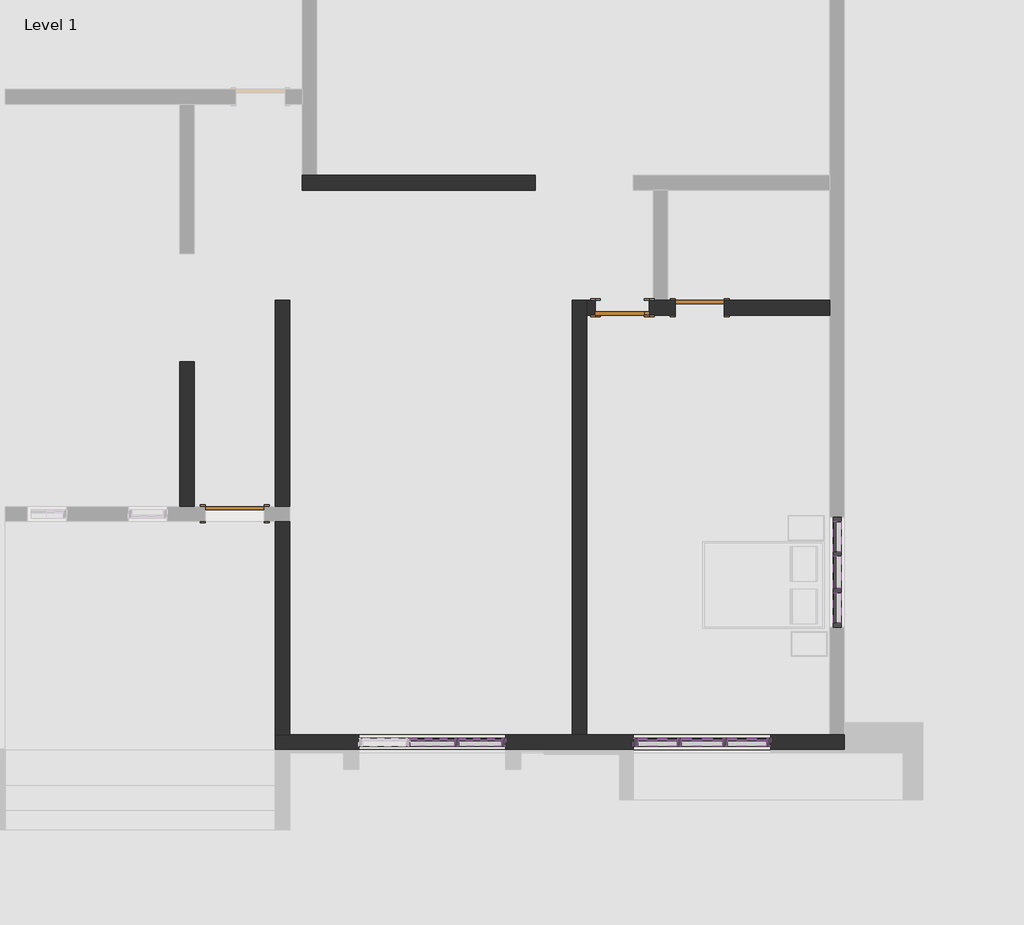
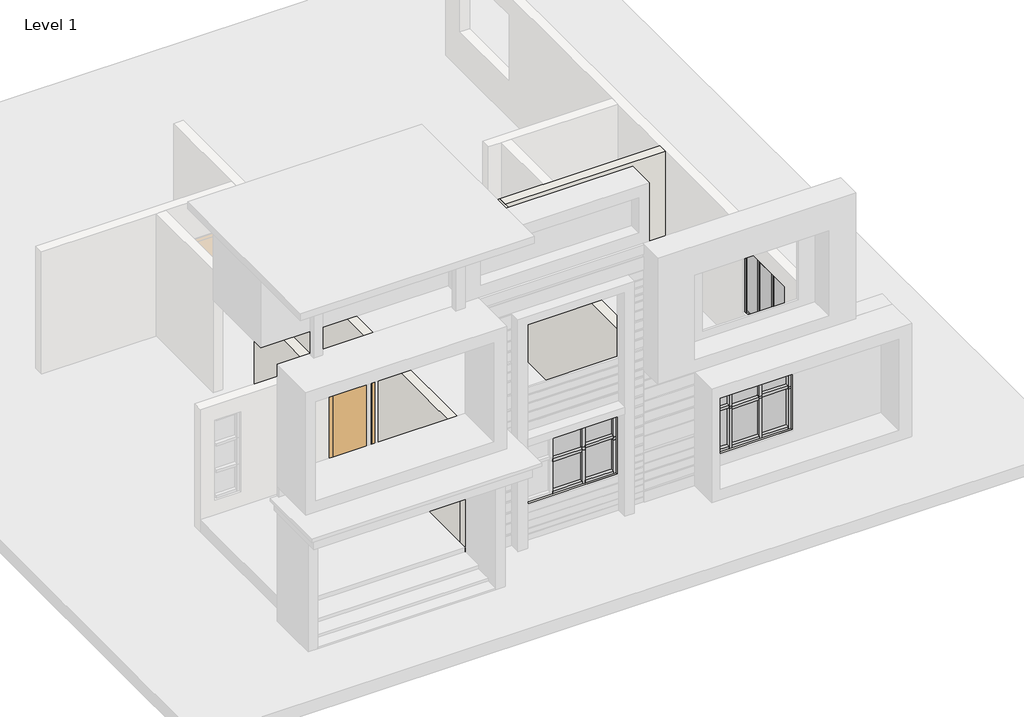
# One storey, part 2 of 3: 43 members, 13 plates, 7 walls, 4 doors.
"""IFC4 building model written with IfcOpenShell, lengths in millimetres."""

from ifc_helpers import new_model, si_unit, origin, origin_with_axes, place, context, project, spatial, polyline, outline, extrude, faceted_brep, transform, mapped, element, save
from components import door_a1484949, door_85036156, door_0ca8825f, member_67dd967c, member_0af91ce1, member_6b0a351e, member_c1cae106, member_3f0e0172, member_5215b92c, member_00d00b53, member_c7c5a8a0, member_eb7364f1, member_b955a9e9, member_5ab2641c, member_2ee2964b, member_c33c434a, member_a6ee1c2c, member_3d7cb871, member_24f36acb, member_06be906d, member_e53b78c9, member_f8dc38bf, member_67d1cd44, member_8f31a534, member_a1cc4565, member_fc709e3d, member_6f38b482, system_panel_glazed_52f1247e, system_panel_glazed_66bb8edf, system_panel_glazed_3a643d3b, system_panel_glazed_b47efb59, system_panel_glazed_21711ca4, system_panel_glazed_687c427d, system_panel_glazed_bb181a04, system_panel_glazed_a28047ed, system_panel_glazed_c0474106, system_panel_glazed_f63241ef

model = new_model("IFC4")

# Units and contexts
model_context = context("Model", 3, world=origin())
ifc_project = project(units=[si_unit("LENGTHUNIT", "METRE", prefix="MILLI")], contexts=[model_context])

# Site, building, storey
site = spatial("IfcSite", under=ifc_project)
building = spatial("IfcBuilding", under=site)
storey = spatial("IfcBuildingStorey", under=building, Name="Level 1", Elevation=0.0)

# Doors
placement = place(None, origin())
door_shape = door_a1484949(model_context)
element("IfcDoor", 1, ObjectType="Single-Flush : 30\" x 80\"", at=placement, inside=storey, context=model_context, shape_type="MappedRepresentation", body=[
    mapped(door_shape, transform((-9027.8261094, -8002.146149, 0.0), x_axis=(-1.0, 0.0, 0.0), y_axis=(0.0, -1.0, 0.0), z_axis=(0.0, 0.0, 1.0))),
])
element("IfcDoor", 2, ObjectType="Single-Flush : 30\" x 80\"", at=placement, inside=storey, context=model_context, shape_type="MappedRepresentation", body=[
    mapped(door_shape, transform((-8951.6261094, -8002.146149, 0.0), x_axis=(-1.0, 0.0, 0.0), y_axis=(0.0, -1.0, 0.0), z_axis=(0.0, 0.0, 1.0))),
])
door_2_shape = door_85036156(model_context)
element("IfcDoor", 3, ObjectType="Single-Flush : 30\" x 80\"", at=placement, inside=storey, context=model_context, shape_type="MappedRepresentation", body=[
    mapped(door_2_shape, transform((-7789.5761094, -8002.146149, 0.0), x_axis=(-1.0, 0.0, 0.0), y_axis=(0.0, -1.0, 0.0), z_axis=(0.0, 0.0, 1.0))),
])
door_3_shape = door_0ca8825f(model_context)
element("IfcDoor", 4, ObjectType="Single-Flush : 36\" x 84\"", at=placement, inside=storey, context=model_context, shape_type="MappedRepresentation", body=[
    mapped(door_3_shape, transform((-15009.5261094, -11202.546149, 355.6), x_axis=(1.0, 0.0, 0.0), y_axis=(0.0, 1.0, 0.0), z_axis=(0.0, 0.0, 1.0))),
])

# Members
member_shape = member_67dd967c(model_context)
element("IfcMember", 5, ObjectType="Rectangular Mullion : 2.5\" x 5\" rectangular", at=placement, inside=storey, context=model_context, shape_type="MappedRepresentation", body=[
    mapped(member_shape, transform((-5655.9761094, -11855.5157064, 2620.512388), x_axis=(0.0, 0.0, 1.0), y_axis=(1.0, 0.0, 0.0), z_axis=(0.0, 1.0, 0.0))),
])
member_2_shape = member_0af91ce1(model_context)
element("IfcMember", 6, ObjectType="Rectangular Mullion : 2.5\" x 5\" rectangular", at=placement, inside=storey, context=model_context, shape_type="MappedRepresentation", body=[
    mapped(member_2_shape, transform((-5655.9761094, -12422.7823731, 2620.512388), x_axis=(0.0, 0.0, 1.0), y_axis=(1.0, 0.0, 0.0), z_axis=(0.0, 1.0, 0.0))),
])
element("IfcMember", 7, ObjectType="Rectangular Mullion : 2.5\" x 5\" rectangular", at=placement, inside=storey, context=model_context, shape_type="MappedRepresentation", body=[
    mapped(member_2_shape, transform((-5655.9761094, -11319.9990397, 2620.512388), x_axis=(0.0, 0.0, 1.0), y_axis=(1.0, 0.0, 0.0), z_axis=(0.0, 1.0, 0.0))),
])
member_3_shape = member_6b0a351e(model_context)
element("IfcMember", 8, ObjectType="Rectangular Mullion : 2.5\" x 5\" rectangular", at=placement, inside=storey, context=model_context, shape_type="MappedRepresentation", body=[
    mapped(member_3_shape, transform((-5655.9761094, -11823.7657064, 945.2248153), x_axis=(0.0, 1.0, 0.0), y_axis=(1.0, 0.0, 0.0), z_axis=(0.0, 0.0, -1.0))),
])
element("IfcMember", 9, ObjectType="Rectangular Mullion : 2.5\" x 5\" rectangular", at=placement, inside=storey, context=model_context, shape_type="MappedRepresentation", body=[
    mapped(member_3_shape, transform((-5655.9761094, -12391.0323731, 945.2248153), x_axis=(0.0, 1.0, 0.0), y_axis=(1.0, 0.0, 0.0), z_axis=(0.0, 0.0, -1.0))),
])
element("IfcMember", 10, ObjectType="Rectangular Mullion : 2.5\" x 5\" rectangular", at=placement, inside=storey, context=model_context, shape_type="MappedRepresentation", body=[
    mapped(member_2_shape, transform((-5655.9761094, -11792.0157064, 945.2248153), x_axis=(0.0, 0.0, -1.0), y_axis=(1.0, 0.0, 0.0), z_axis=(0.0, -1.0, 0.0))),
])
element("IfcMember", 11, ObjectType="Rectangular Mullion : 2.5\" x 5\" rectangular", at=placement, inside=storey, context=model_context, shape_type="MappedRepresentation", body=[
    mapped(member_2_shape, transform((-5655.9761094, -12894.7990397, 945.2248153), x_axis=(0.0, 0.0, -1.0), y_axis=(1.0, 0.0, 0.0), z_axis=(0.0, -1.0, 0.0))),
])
element("IfcMember", 12, ObjectType="Rectangular Mullion : 2.5\" x 5\" rectangular", at=placement, inside=storey, context=model_context, shape_type="MappedRepresentation", body=[
    mapped(member_shape, transform((-5655.9761094, -12359.2823731, 945.2248153), x_axis=(0.0, 0.0, -1.0), y_axis=(1.0, 0.0, 0.0), z_axis=(0.0, -1.0, 0.0))),
])
member_4_shape = member_c1cae106(model_context)
element("IfcMember", 13, ObjectType="Rectangular Mullion : 2.5\" x 5\" rectangular", at=placement, inside=storey, context=model_context, shape_type="MappedRepresentation", body=[
    mapped(member_4_shape, transform((-5655.9761094, -11256.4990397, 945.2248153), x_axis=(0.0, 1.0, 0.0), y_axis=(1.0, 0.0, 0.0), z_axis=(0.0, 0.0, -1.0))),
])
element("IfcMember", 14, ObjectType="Rectangular Mullion : 2.5\" x 5\" rectangular", at=placement, inside=storey, context=model_context, shape_type="MappedRepresentation", body=[
    mapped(member_4_shape, transform((-5655.9761094, -12958.2990397, 2620.512388), x_axis=(0.0, -1.0, 0.0), y_axis=(1.0, 0.0, 0.0), z_axis=(0.0, 0.0, 1.0))),
])
member_5_shape = member_3f0e0172(model_context)
element("IfcMember", 15, ObjectType="Rectangular Mullion : 2.5\" x 5\" rectangular", at=placement, inside=storey, context=model_context, shape_type="MappedRepresentation", body=[
    mapped(member_5_shape, transform((-8139.2627168, -14745.846149, 2528.3677735), x_axis=(0.0, 0.0, 1.0), y_axis=(0.0, -1.0, 0.0), z_axis=(1.0, 0.0, 0.0))),
])
element("IfcMember", 16, ObjectType="Rectangular Mullion : 2.5\" x 5\" rectangular", at=placement, inside=storey, context=model_context, shape_type="MappedRepresentation", body=[
    mapped(member_5_shape, transform((-6748.6127168, -14745.846149, 2528.3677735), x_axis=(0.0, 0.0, 1.0), y_axis=(0.0, -1.0, 0.0), z_axis=(1.0, 0.0, 0.0))),
])
element("IfcMember", 17, ObjectType="Rectangular Mullion : 2.5\" x 5\" rectangular", at=placement, inside=storey, context=model_context, shape_type="MappedRepresentation", body=[
    mapped(member_5_shape, transform((-7364.5627168, -14745.846149, 537.8317429), x_axis=(0.0, 0.0, -1.0), y_axis=(0.0, -1.0, 0.0), z_axis=(-1.0, 0.0, 0.0))),
])
element("IfcMember", 18, ObjectType="Rectangular Mullion : 2.5\" x 5\" rectangular", at=placement, inside=storey, context=model_context, shape_type="MappedRepresentation", body=[
    mapped(member_5_shape, transform((-8755.2127168, -14745.846149, 537.8317429), x_axis=(0.0, 0.0, -1.0), y_axis=(0.0, -1.0, 0.0), z_axis=(-1.0, 0.0, 0.0))),
])
member_6_shape = member_5215b92c(model_context)
element("IfcMember", 19, ObjectType="Rectangular Mullion : 2.5\" x 5\" rectangular", at=placement, inside=storey, context=model_context, shape_type="MappedRepresentation", body=[
    mapped(member_6_shape, transform((-7428.0627168, -14745.846149, 2528.3677735), x_axis=(0.0, 0.0, 1.0), y_axis=(0.0, -1.0, 0.0), z_axis=(1.0, 0.0, 0.0))),
])
element("IfcMember", 20, ObjectType="Rectangular Mullion : 2.5\" x 5\" rectangular", at=placement, inside=storey, context=model_context, shape_type="MappedRepresentation", body=[
    mapped(member_6_shape, transform((-8075.7627168, -14745.846149, 537.8317429), x_axis=(0.0, 0.0, -1.0), y_axis=(0.0, -1.0, 0.0), z_axis=(-1.0, 0.0, 0.0))),
])
member_7_shape = member_00d00b53(model_context)
element("IfcMember", 21, ObjectType="Rectangular Mullion : 2.5\" x 5\" rectangular", at=placement, inside=storey, context=model_context, shape_type="MappedRepresentation", body=[
    mapped(member_7_shape, transform((-11561.9127168, -14745.846149, 1704.2081862), x_axis=(1.0, 0.0, 0.0), y_axis=(0.0, -1.0, 0.0), z_axis=(0.0, 0.0, -1.0))),
])
member_8_shape = member_c7c5a8a0(model_context)
element("IfcMember", 22, ObjectType="Rectangular Mullion : 2.5\" x 5\" rectangular", at=placement, inside=storey, context=model_context, shape_type="MappedRepresentation", body=[
    mapped(member_8_shape, transform((-11593.6627168, -14745.846149, 1704.2081862), x_axis=(0.0, 0.0, 1.0), y_axis=(0.0, -1.0, 0.0), z_axis=(1.0, 0.0, 0.0))),
])
member_9_shape = member_eb7364f1(model_context)
element("IfcMember", 23, ObjectType="Rectangular Mullion : 2.5\" x 5\" rectangular", at=placement, inside=storey, context=model_context, shape_type="MappedRepresentation", body=[
    mapped(member_9_shape, transform((-11561.9127168, -14745.846149, 1780.4081862), x_axis=(1.0, 0.0, 0.0), y_axis=(0.0, -1.0, 0.0), z_axis=(0.0, 0.0, -1.0))),
])
member_10_shape = member_b955a9e9(model_context)
element("IfcMember", 24, ObjectType="Rectangular Mullion : 2.5\" x 5\" rectangular", at=placement, inside=storey, context=model_context, shape_type="MappedRepresentation", body=[
    mapped(member_10_shape, transform((-11593.6627168, -14745.846149, 2536.7442955), x_axis=(0.0, 0.0, 1.0), y_axis=(0.0, -1.0, 0.0), z_axis=(1.0, 0.0, 0.0))),
])
member_11_shape = member_5ab2641c(model_context)
element("IfcMember", 25, ObjectType="Rectangular Mullion : 2.5\" x 5\" rectangular", at=placement, inside=storey, context=model_context, shape_type="MappedRepresentation", body=[
    mapped(member_11_shape, transform((-11561.9127168, -14745.846149, 871.6720769), x_axis=(1.0, 0.0, 0.0), y_axis=(0.0, -1.0, 0.0), z_axis=(0.0, 0.0, -1.0))),
])
element("IfcMember", 26, ObjectType="Rectangular Mullion : 2.5\" x 5\" rectangular", at=placement, inside=storey, context=model_context, shape_type="MappedRepresentation", body=[
    mapped(member_10_shape, transform((-12292.1627168, -14745.846149, 871.6720769), x_axis=(0.0, 0.0, -1.0), y_axis=(0.0, -1.0, 0.0), z_axis=(-1.0, 0.0, 0.0))),
])
member_12_shape = member_2ee2964b(model_context)
element("IfcMember", 27, ObjectType="Rectangular Mullion : 2.5\" x 5\" rectangular", at=placement, inside=storey, context=model_context, shape_type="MappedRepresentation", body=[
    mapped(member_12_shape, transform((-10863.4127168, -14745.846149, 1780.4081862), x_axis=(0.0, 0.0, 1.0), y_axis=(0.0, -1.0, 0.0), z_axis=(1.0, 0.0, 0.0))),
])
member_13_shape = member_c33c434a(model_context)
element("IfcMember", 28, ObjectType="Rectangular Mullion : 2.5\" x 5\" rectangular", at=placement, inside=storey, context=model_context, shape_type="MappedRepresentation", body=[
    mapped(member_13_shape, transform((-10863.4127168, -14745.846149, 2536.7442955), x_axis=(0.0, 0.0, 1.0), y_axis=(0.0, -1.0, 0.0), z_axis=(1.0, 0.0, 0.0))),
])
element("IfcMember", 29, ObjectType="Rectangular Mullion : 2.5\" x 5\" rectangular", at=placement, inside=storey, context=model_context, shape_type="MappedRepresentation", body=[
    mapped(member_13_shape, transform((-11530.1627168, -14745.846149, 871.6720769), x_axis=(0.0, 0.0, -1.0), y_axis=(0.0, -1.0, 0.0), z_axis=(-1.0, 0.0, 0.0))),
])
member_14_shape = member_a6ee1c2c(model_context)
element("IfcMember", 30, ObjectType="Rectangular Mullion : 2.5\" x 5\" rectangular", at=placement, inside=storey, context=model_context, shape_type="MappedRepresentation", body=[
    mapped(member_14_shape, transform((-10799.9127168, -14745.846149, 1780.4081862), x_axis=(1.0, 0.0, 0.0), y_axis=(0.0, -1.0, 0.0), z_axis=(0.0, 0.0, -1.0))),
])
member_15_shape = member_3d7cb871(model_context)
element("IfcMember", 31, ObjectType="Rectangular Mullion : 2.5\" x 5\" rectangular", at=placement, inside=storey, context=model_context, shape_type="MappedRepresentation", body=[
    mapped(member_15_shape, transform((-10799.9127168, -14745.846149, 1704.2081862), x_axis=(1.0, 0.0, 0.0), y_axis=(0.0, -1.0, 0.0), z_axis=(0.0, 0.0, -1.0))),
])
member_16_shape = member_24f36acb(model_context)
element("IfcMember", 32, ObjectType="Rectangular Mullion : 2.5\" x 5\" rectangular", at=placement, inside=storey, context=model_context, shape_type="MappedRepresentation", body=[
    mapped(member_16_shape, transform((-10799.9127168, -14745.846149, 871.6720769), x_axis=(1.0, 0.0, 0.0), y_axis=(0.0, -1.0, 0.0), z_axis=(0.0, 0.0, -1.0))),
])
member_17_shape = member_06be906d(model_context)
element("IfcMember", 33, ObjectType="Rectangular Mullion : 2.5\" x 5\" rectangular", at=placement, inside=storey, context=model_context, shape_type="MappedRepresentation", body=[
    mapped(member_17_shape, transform((-7396.3127168, -14745.846149, 1533.0997582), x_axis=(1.0, 0.0, 0.0), y_axis=(0.0, -1.0, 0.0), z_axis=(0.0, 0.0, -1.0))),
])
element("IfcMember", 34, ObjectType="Rectangular Mullion : 2.5\" x 5\" rectangular", at=placement, inside=storey, context=model_context, shape_type="MappedRepresentation", body=[
    mapped(member_17_shape, transform((-8107.5127168, -14745.846149, 1533.0997582), x_axis=(1.0, 0.0, 0.0), y_axis=(0.0, -1.0, 0.0), z_axis=(0.0, 0.0, -1.0))),
])
member_18_shape = member_e53b78c9(model_context)
element("IfcMember", 35, ObjectType="Rectangular Mullion : 2.5\" x 5\" rectangular", at=placement, inside=storey, context=model_context, shape_type="MappedRepresentation", body=[
    mapped(member_18_shape, transform((-7428.0627168, -14745.846149, 1533.0997582), x_axis=(0.0, 0.0, 1.0), y_axis=(0.0, -1.0, 0.0), z_axis=(1.0, 0.0, 0.0))),
])
member_19_shape = member_f8dc38bf(model_context)
element("IfcMember", 36, ObjectType="Rectangular Mullion : 2.5\" x 5\" rectangular", at=placement, inside=storey, context=model_context, shape_type="MappedRepresentation", body=[
    mapped(member_19_shape, transform((-6748.6127168, -14745.846149, 1583.8997582), x_axis=(0.0, 0.0, 1.0), y_axis=(0.0, -1.0, 0.0), z_axis=(1.0, 0.0, 0.0))),
])
element("IfcMember", 37, ObjectType="Rectangular Mullion : 2.5\" x 5\" rectangular", at=placement, inside=storey, context=model_context, shape_type="MappedRepresentation", body=[
    mapped(member_19_shape, transform((-8139.2627168, -14745.846149, 1583.8997582), x_axis=(0.0, 0.0, 1.0), y_axis=(0.0, -1.0, 0.0), z_axis=(1.0, 0.0, 0.0))),
])
member_20_shape = member_67d1cd44(model_context)
element("IfcMember", 38, ObjectType="Rectangular Mullion : 2.5\" x 5\" rectangular", at=placement, inside=storey, context=model_context, shape_type="MappedRepresentation", body=[
    mapped(member_20_shape, transform((-8818.7127168, -14745.846149, 1583.8997582), x_axis=(-1.0, 0.0, 0.0), y_axis=(0.0, -1.0, 0.0), z_axis=(0.0, 0.0, 1.0))),
])
member_21_shape = member_8f31a534(model_context)
element("IfcMember", 39, ObjectType="Rectangular Mullion : 2.5\" x 5\" rectangular", at=placement, inside=storey, context=model_context, shape_type="MappedRepresentation", body=[
    mapped(member_21_shape, transform((-7396.3127168, -14745.846149, 537.8317429), x_axis=(1.0, 0.0, 0.0), y_axis=(0.0, -1.0, 0.0), z_axis=(0.0, 0.0, -1.0))),
])
element("IfcMember", 40, ObjectType="Rectangular Mullion : 2.5\" x 5\" rectangular", at=placement, inside=storey, context=model_context, shape_type="MappedRepresentation", body=[
    mapped(member_21_shape, transform((-8107.5127168, -14745.846149, 537.8317429), x_axis=(1.0, 0.0, 0.0), y_axis=(0.0, -1.0, 0.0), z_axis=(0.0, 0.0, -1.0))),
])
member_22_shape = member_a1cc4565(model_context)
element("IfcMember", 41, ObjectType="Rectangular Mullion : 2.5\" x 5\" rectangular", at=placement, inside=storey, context=model_context, shape_type="MappedRepresentation", body=[
    mapped(member_22_shape, transform((-8818.7127168, -14745.846149, 1533.0997582), x_axis=(-1.0, 0.0, 0.0), y_axis=(0.0, -1.0, 0.0), z_axis=(0.0, 0.0, 1.0))),
])
element("IfcMember", 42, ObjectType="Rectangular Mullion : 2.5\" x 5\" rectangular", at=placement, inside=storey, context=model_context, shape_type="MappedRepresentation", body=[
    mapped(member_20_shape, transform((-6685.1127168, -14745.846149, 1533.0997582), x_axis=(1.0, 0.0, 0.0), y_axis=(0.0, -1.0, 0.0), z_axis=(0.0, 0.0, -1.0))),
])
element("IfcMember", 43, ObjectType="Rectangular Mullion : 2.5\" x 5\" rectangular", at=placement, inside=storey, context=model_context, shape_type="MappedRepresentation", body=[
    mapped(member_22_shape, transform((-6685.1127168, -14745.846149, 537.8317429), x_axis=(1.0, 0.0, 0.0), y_axis=(0.0, -1.0, 0.0), z_axis=(0.0, 0.0, -1.0))),
])
member_23_shape = member_fc709e3d(model_context)
element("IfcMember", 44, ObjectType="Rectangular Mullion : 2.5\" x 5\" rectangular", at=placement, inside=storey, context=model_context, shape_type="MappedRepresentation", body=[
    mapped(member_23_shape, transform((-7396.3127168, -14745.846149, 1583.8997582), x_axis=(1.0, 0.0, 0.0), y_axis=(0.0, -1.0, 0.0), z_axis=(0.0, 0.0, -1.0))),
])
element("IfcMember", 45, ObjectType="Rectangular Mullion : 2.5\" x 5\" rectangular", at=placement, inside=storey, context=model_context, shape_type="MappedRepresentation", body=[
    mapped(member_23_shape, transform((-8107.5127168, -14745.846149, 1583.8997582), x_axis=(1.0, 0.0, 0.0), y_axis=(0.0, -1.0, 0.0), z_axis=(0.0, 0.0, -1.0))),
])
member_24_shape = member_6f38b482(model_context)
element("IfcMember", 46, ObjectType="Rectangular Mullion : 2.5\" x 5\" rectangular", at=placement, inside=storey, context=model_context, shape_type="MappedRepresentation", body=[
    mapped(member_24_shape, transform((-8818.7127168, -14745.846149, 2528.3677735), x_axis=(-1.0, 0.0, 0.0), y_axis=(0.0, -1.0, 0.0), z_axis=(0.0, 0.0, 1.0))),
])
element("IfcMember", 47, ObjectType="Rectangular Mullion : 2.5\" x 5\" rectangular", at=placement, inside=storey, context=model_context, shape_type="MappedRepresentation", body=[
    mapped(member_24_shape, transform((-6685.1127168, -14745.846149, 1583.8997582), x_axis=(1.0, 0.0, 0.0), y_axis=(0.0, -1.0, 0.0), z_axis=(0.0, 0.0, -1.0))),
])

# Plates
system_panel_glazed_shape = system_panel_glazed_52f1247e(model_context)
element("IfcPlate", 48, ObjectType="System Panel : Glazed", at=placement, inside=storey, context=model_context, shape_type="MappedRepresentation", body=[
    mapped(system_panel_glazed_shape, transform((-5655.9761094, -12658.7907064, 1008.7248153), x_axis=(0.0, 1.0, 0.0), y_axis=(-1.0, 0.0, 0.0), z_axis=(0.0, 0.0, 1.0))),
])
element("IfcPlate", 49, ObjectType="System Panel : Glazed", at=placement, inside=storey, context=model_context, shape_type="MappedRepresentation", body=[
    mapped(system_panel_glazed_shape, transform((-5655.9761094, -11556.0073731, 1008.7248153), x_axis=(0.0, 1.0, 0.0), y_axis=(-1.0, 0.0, 0.0), z_axis=(0.0, 0.0, 1.0))),
])
system_panel_glazed_2_shape = system_panel_glazed_66bb8edf(model_context)
element("IfcPlate", 50, ObjectType="System Panel : Glazed", at=placement, inside=storey, context=model_context, shape_type="MappedRepresentation", body=[
    mapped(system_panel_glazed_2_shape, transform((-5655.9761094, -12107.3990397, 1008.7248153), x_axis=(0.0, 1.0, 0.0), y_axis=(-1.0, 0.0, 0.0), z_axis=(0.0, 0.0, 1.0))),
])
system_panel_glazed_3_shape = system_panel_glazed_3a643d3b(model_context)
element("IfcPlate", 51, ObjectType="System Panel : Glazed", at=placement, inside=storey, context=model_context, shape_type="MappedRepresentation", body=[
    mapped(system_panel_glazed_3_shape, transform((-11942.9127168, -14745.846149, 1735.9581862), x_axis=(1.0, 0.0, 0.0), y_axis=(0.0, 1.0, 0.0), z_axis=(0.0, 0.0, 1.0))),
])
system_panel_glazed_4_shape = system_panel_glazed_b47efb59(model_context)
element("IfcPlate", 52, ObjectType="System Panel : Glazed", at=placement, inside=storey, context=model_context, shape_type="MappedRepresentation", body=[
    mapped(system_panel_glazed_4_shape, transform((-11942.9127168, -14745.846149, 935.1720769), x_axis=(1.0, 0.0, 0.0), y_axis=(0.0, 1.0, 0.0), z_axis=(0.0, 0.0, 1.0))),
])
system_panel_glazed_5_shape = system_panel_glazed_21711ca4(model_context)
element("IfcPlate", 53, ObjectType="System Panel : Glazed", at=placement, inside=storey, context=model_context, shape_type="MappedRepresentation", body=[
    mapped(system_panel_glazed_5_shape, transform((-11196.7877168, -14745.846149, 935.1720769), x_axis=(1.0, 0.0, 0.0), y_axis=(0.0, 1.0, 0.0), z_axis=(0.0, 0.0, 1.0))),
])
system_panel_glazed_6_shape = system_panel_glazed_687c427d(model_context)
element("IfcPlate", 54, ObjectType="System Panel : Glazed", at=placement, inside=storey, context=model_context, shape_type="MappedRepresentation", body=[
    mapped(system_panel_glazed_6_shape, transform((-11196.7877168, -14745.846149, 1812.1581862), x_axis=(1.0, 0.0, 0.0), y_axis=(0.0, 1.0, 0.0), z_axis=(0.0, 0.0, 1.0))),
])
system_panel_glazed_7_shape = system_panel_glazed_bb181a04(model_context)
element("IfcPlate", 55, ObjectType="System Panel : Glazed", at=placement, inside=storey, context=model_context, shape_type="MappedRepresentation", body=[
    mapped(system_panel_glazed_7_shape, transform((-8447.2377168, -14745.846149, 601.3317429), x_axis=(1.0, 0.0, 0.0), y_axis=(0.0, 1.0, 0.0), z_axis=(0.0, 0.0, 1.0))),
])
element("IfcPlate", 56, ObjectType="System Panel : Glazed", at=placement, inside=storey, context=model_context, shape_type="MappedRepresentation", body=[
    mapped(system_panel_glazed_7_shape, transform((-7056.5877168, -14745.846149, 601.3317429), x_axis=(1.0, 0.0, 0.0), y_axis=(0.0, 1.0, 0.0), z_axis=(0.0, 0.0, 1.0))),
])
system_panel_glazed_8_shape = system_panel_glazed_a28047ed(model_context)
element("IfcPlate", 57, ObjectType="System Panel : Glazed", at=placement, inside=storey, context=model_context, shape_type="MappedRepresentation", body=[
    mapped(system_panel_glazed_8_shape, transform((-7751.9127168, -14745.846149, 601.3317429), x_axis=(1.0, 0.0, 0.0), y_axis=(0.0, 1.0, 0.0), z_axis=(0.0, 0.0, 1.0))),
])
system_panel_glazed_9_shape = system_panel_glazed_c0474106(model_context)
element("IfcPlate", 58, ObjectType="System Panel : Glazed", at=placement, inside=storey, context=model_context, shape_type="MappedRepresentation", body=[
    mapped(system_panel_glazed_9_shape, transform((-7751.9127168, -14745.846149, 1564.8497582), x_axis=(1.0, 0.0, 0.0), y_axis=(0.0, 1.0, 0.0), z_axis=(0.0, 0.0, 1.0))),
])
system_panel_glazed_10_shape = system_panel_glazed_f63241ef(model_context)
element("IfcPlate", 59, ObjectType="System Panel : Glazed", at=placement, inside=storey, context=model_context, shape_type="MappedRepresentation", body=[
    mapped(system_panel_glazed_10_shape, transform((-8447.2377168, -14745.846149, 1615.6497582), x_axis=(1.0, 0.0, 0.0), y_axis=(0.0, 1.0, 0.0), z_axis=(0.0, 0.0, 1.0))),
])
element("IfcPlate", 60, ObjectType="System Panel : Glazed", at=placement, inside=storey, context=model_context, shape_type="MappedRepresentation", body=[
    mapped(system_panel_glazed_10_shape, transform((-7056.5877168, -14745.846149, 1615.6497582), x_axis=(1.0, 0.0, 0.0), y_axis=(0.0, 1.0, 0.0), z_axis=(0.0, 0.0, 1.0))),
])

# Walls
element("IfcWall", 61, ObjectType="9\"", at=placement, inside=storey, context=model_context, shape_type="SweptSolid", body=[
    extrude(outline(polyline([(-14380.8761094, -14631.546149), (-14380.8761094, -11316.846149), (-14152.2761094, -11316.846149), (-14152.2761094, -14631.546149), (-14380.8761094, -14631.546149)])), origin_with_axes(), (0.0, 0.0, 1.0), 3048.0),
])
element("IfcWall", 62, ObjectType="9\"", at=placement, inside=storey, context=model_context, shape_type="SweptSolid", body=[
    extrude(outline(polyline([(-14152.2761094, -7887.846149), (-14152.2761094, -11088.246149), (-14380.8761094, -11088.246149), (-14380.8761094, -7887.846149), (-14152.2761094, -7887.846149)])), origin_with_axes(), (0.0, 0.0, 1.0), 3048.0),
])
element("IfcWall", 63, ObjectType="9\"", at=placement, inside=storey, context=model_context, shape_type="Brep", body=[
    faceted_brep([(-9542.1761094, -14631.546149, 0.0), (-9542.1761094, -8116.446149, 0.0), (-9542.1761094, -7887.846149, 0.0), (-9542.1761094, -7887.846149, 3048.0), (-9542.1761094, -8116.446149, 3048.0), (-9542.1761094, -14631.546149, 3048.0), (-9770.7761094, -14631.546149, 0.0), (-9770.7761094, -14631.546149, 3048.0), (-9770.7761094, -7887.846149, 3048.0), (-9770.7761094, -7887.846149, 0.0)], [[[0, 1, 2, 3, 4, 5]], [[6, 7, 8, 9]], [[2, 1, 0, 6, 9]], [[5, 4, 3, 8, 7]], [[0, 5, 7, 6]], [[3, 2, 9, 8]]]),
])
element("IfcWall", 64, ObjectType="9\"", at=placement, inside=storey, context=model_context, shape_type="Brep", body=[
    faceted_brep([(-8570.6261094, -8116.446149, 0.0), (-8170.5761094, -8116.446149, 0.0), (-8170.5761094, -8116.446149, 2032.0), (-7408.5761094, -8116.446149, 2032.0), (-7408.5761094, -8116.446149, 0.0), (-5770.2761094, -8116.446149, 0.0), (-5770.2761094, -8116.446149, 3048.0), (-9542.1761094, -8116.446149, 3048.0), (-9542.1761094, -8116.446149, 0.0), (-9408.8261094, -8116.446149, 0.0), (-9408.8261094, -8116.446149, 2032.0), (-8570.6261094, -8116.446149, 2032.0), (-8170.5761094, -7887.846149, 2032.0), (-8170.5761094, -7887.846149, 0.0), (-8284.8761094, -7887.846149, 0.0), (-8513.4761094, -7887.846149, 0.0), (-8570.6261094, -7887.846149, 0.0), (-8570.6261094, -7887.846149, 2032.0), (-9408.8261094, -7887.846149, 2032.0), (-9408.8261094, -7887.846149, 0.0), (-9542.1761094, -7887.846149, 0.0), (-9542.1761094, -7887.846149, 3048.0), (-8513.4761094, -7887.846149, 3048.0), (-8284.8761094, -7887.846149, 3048.0), (-5770.2761094, -7887.846149, 3048.0), (-5770.2761094, -7887.846149, 0.0), (-7408.5761094, -7887.846149, 0.0), (-7408.5761094, -7887.846149, 2032.0)], [[[0, 1, 2, 3, 4, 5, 6, 7, 8, 9, 10, 11]], [[12, 13, 14, 15, 16, 17, 18, 19, 20, 21, 22, 23, 24, 25, 26, 27]], [[8, 20, 19, 9]], [[26, 25, 5, 4]], [[16, 15, 14, 13, 1, 0]], [[7, 6, 24, 23, 22, 21]], [[8, 7, 21, 20]], [[6, 5, 25, 24]], [[10, 9, 19, 18]], [[10, 18, 17, 11]], [[11, 17, 16, 0]], [[2, 1, 13, 12]], [[3, 2, 12, 27]], [[4, 3, 27, 26]]]),
])
element("IfcWall", 65, ObjectType="9\"", at=placement, inside=storey, context=model_context, shape_type="SweptSolid", body=[
    extrude(outline(polyline([(-15866.7761094, -11088.246149), (-15866.7761094, -8840.346149), (-15638.1761094, -8840.346149), (-15638.1761094, -11088.246149), (-15866.7761094, -11088.246149)])), origin_with_axes(), (0.0, 0.0, 1.0), 3048.0),
])
element("IfcWall", 66, ObjectType="9\"", at=placement, inside=storey, context=model_context, shape_type="Brep", body=[
    faceted_brep([(-10342.7127168, -5944.746149, 0.0), (-13733.6127168, -5944.746149, 0.0), (-13962.2127168, -5944.746149, 0.0), (-13962.2127168, -5944.746149, 3048.0), (-13733.6127168, -5944.746149, 3048.0), (-10342.7127168, -5944.746149, 3048.0), (-10342.7127168, -6173.346149, 0.0), (-10342.7127168, -6173.346149, 3048.0), (-13962.2127168, -6173.346149, 3048.0), (-13962.2127168, -6173.346149, 0.0)], [[[0, 1, 2, 3, 4, 5]], [[6, 7, 8, 9]], [[2, 1, 0, 6, 9]], [[5, 4, 3, 8, 7]], [[0, 5, 7, 6]], [[3, 2, 9, 8]]]),
])
element("IfcWall", 67, ObjectType="9\"", at=placement, inside=storey, context=model_context, shape_type="Brep", body=[
    faceted_brep([(-14380.8761094, -14860.146149, 0.0), (-5541.6761094, -14860.146149, 0.0), (-5541.6761094, -14860.146149, 3048.0), (-14380.8761094, -14860.146149, 3048.0), (-13085.9127168, -14860.146149, 871.6720769), (-13085.9127168, -14860.146149, 2536.7442955), (-10799.9127168, -14860.146149, 2536.7442955), (-10799.9127168, -14860.146149, 871.6720769), (-8818.7127168, -14860.146149, 537.8317429), (-8818.7127168, -14860.146149, 2528.3677735), (-6685.1127168, -14860.146149, 2528.3677735), (-6685.1127168, -14860.146149, 537.8317429), (-5541.6761094, -14631.546149, 0.0), (-5770.2761094, -14631.546149, 0.0), (-9542.1761094, -14631.546149, 0.0), (-9770.7761094, -14631.546149, 0.0), (-14152.2761094, -14631.546149, 0.0), (-14380.8761094, -14631.546149, 0.0), (-14380.8761094, -14631.546149, 3048.0), (-14152.2761094, -14631.546149, 3048.0), (-9770.7761094, -14631.546149, 3048.0), (-9542.1761094, -14631.546149, 3048.0), (-5770.2761094, -14631.546149, 3048.0), (-5541.6761094, -14631.546149, 3048.0), (-13085.9127168, -14631.546149, 2536.7442955), (-13085.9127168, -14631.546149, 871.6720769), (-10799.9127168, -14631.546149, 871.6720769), (-10799.9127168, -14631.546149, 2536.7442955), (-8818.7127168, -14631.546149, 2528.3677735), (-8818.7127168, -14631.546149, 537.8317429), (-6685.1127168, -14631.546149, 537.8317429), (-6685.1127168, -14631.546149, 2528.3677735)], [[[0, 1, 2, 3], [4, 5, 6, 7], [8, 9, 10, 11]], [[12, 13, 14, 15, 16, 17, 18, 19, 20, 21, 22, 23], [24, 25, 26, 27], [28, 29, 30, 31]], [[1, 0, 17, 16, 15, 14, 13, 12]], [[3, 2, 23, 22, 21, 20, 19, 18]], [[0, 3, 18, 17]], [[2, 1, 12, 23]], [[24, 5, 4, 25]], [[5, 24, 27, 6]], [[6, 27, 26, 7]], [[25, 4, 7, 26]], [[8, 29, 28, 9]], [[9, 28, 31, 10]], [[10, 31, 30, 11]], [[29, 8, 11, 30]]]),
])

save(model, "model.ifc")

# Revit data of these elements
# Type "Single-Flush : 30\" x 80\""
#   Type Mark = "5"
#   Construction Type Id = "MDOOR"
#   Assembly Code = "C1020"
#   Analytic Construction = "Metal"
#   Thickness = 0' - 2"
#   Heat Transfer Coefficient (U) = 0.651978 BTU/(h·ft²·°F)
#   Height = 6' - 8"
#   Trim Projection Ext = 0' - 1"
#   Trim Projection Int = 0' - 1"
#   Trim Width = 0' - 3"
#   Width = 2' - 6"
#   Define Thermal Properties by = 1
#   Define Thermal Properties by = 1
#   Door Material = Door - Panel
#   Frame Material = Door - Frame
#   Visual Light Transmittance = 0
#   Solar Heat Gain Coefficient = 0
#   Function = (empty or 0)
#   Wall Closure = (empty or 0)
# Type "Single-Flush : 36\" x 84\""
#   Type Mark = "1"
#   Construction Type Id = "MDOOR"
#   Assembly Code = "C1020"
#   Analytic Construction = "Metal"
#   Thickness = 0' - 2"
#   Heat Transfer Coefficient (U) = 0.651978 BTU/(h·ft²·°F)
#   Height = 7' - 0"
#   Trim Projection Ext = 0' - 1"
#   Trim Projection Int = 0' - 1"
#   Trim Width = 0' - 3"
#   Width = 3' - 0"
#   Define Thermal Properties by = 1
#   Define Thermal Properties by = 1
#   Door Material = Door - Panel
#   Frame Material = Door - Frame
#   Visual Light Transmittance = 0
#   Solar Heat Gain Coefficient = 0
#   Function = (empty or 0)
#   Wall Closure = (empty or 0)
# Type "Rectangular Mullion : 2.5\" x 5\" rectangular"
#   built-in parameter 1007304 = 0.416667 (stored number, unit not read)
#   built-in parameter 1007301 = 0.104167 (stored number, unit not read)
#   built-in parameter 1007300 = 0.104167 (stored number, unit not read)
# Type "System Panel : Glazed"
#   Construction Type Id = "GSP4R"
#   Analytic Construction = "1/8 in Pilkington single glazing"
#   Visual Light Transmittance = 0.9
#   Solar Heat Gain Coefficient = 0.86
#   Heat Transfer Coefficient (U) = 1.18115 BTU/(h·ft²·°F)
#   Define Thermal Properties by = 1
# Type "9\""
#   Assembly Code = "B2010"
#   Layers, outside or top first: 0' - 9" no material (function 1)
# Elements 1, 2, 3 (IfcDoor, "Single-Flush : 30\" x 80\"")
#   Phase Created = New Construction
#   Materials on its faces: "Door - Frame", "Door - Panel"
# Element 4 (IfcDoor, "Single-Flush : 36\" x 84\"")
#   Phase Created = New Construction
#   Materials on its faces: "Door - Frame", "Door - Panel"
# Elements 5, 6, 7, 8, 9, 10, 11, 12, 13, 14, 15, 16, 17, 18, 19, 20, 21, 22, 23, 24, 25, 26, 27, 28, 29, 30, 31, 32, 33, 34, 35, 36, 37, 38, 39, 40, 41, 42, 43, 44, 45, 46, 47 (IfcMember, "Rectangular Mullion : 2.5\" x 5\" rectangular")
#   Phase Created = New Construction
#   Materials on its faces: "Aluminum"
# Elements 48, 49, 50, 51, 52, 53, 54, 55, 56, 57, 58, 59, 60 (IfcPlate, "System Panel : Glazed")
#   Phase Created = New Construction
#   Materials on its faces: "Glass"
# Elements 61, 62, 63, 64, 65, 66, 67 (IfcWall, "9\"")
#   Top Offset = 0' - 0"
#   Base Offset = 0' - 0"
#   Unconnected Height = 10' - 0"
#   wall height = 10' - 0"
#   Phase Created = New Construction
#   Base Constraint = Level 1
#   Materials on its faces: "Default Wall"
# Materials
#   "Door - Panel": class "Wood", colour RGB 210 159 95, transparency 0, Cost = 0
#   "Door - Frame": colour RGB 118 70 51, transparency 0, Cost = 0
#   "Aluminum": class "Metal", colour RGB 247 247 247, transparency 0, Description = "Aluminum 6061", Cost = 0
#   "Glass": class "Glass", colour RGB 0 128 192, transparency 0.75, Description = "Soda Lime Glass", Cost = 0
#   "Default Wall": colour RGB 128 128 128, transparency 0, Cost = 0
